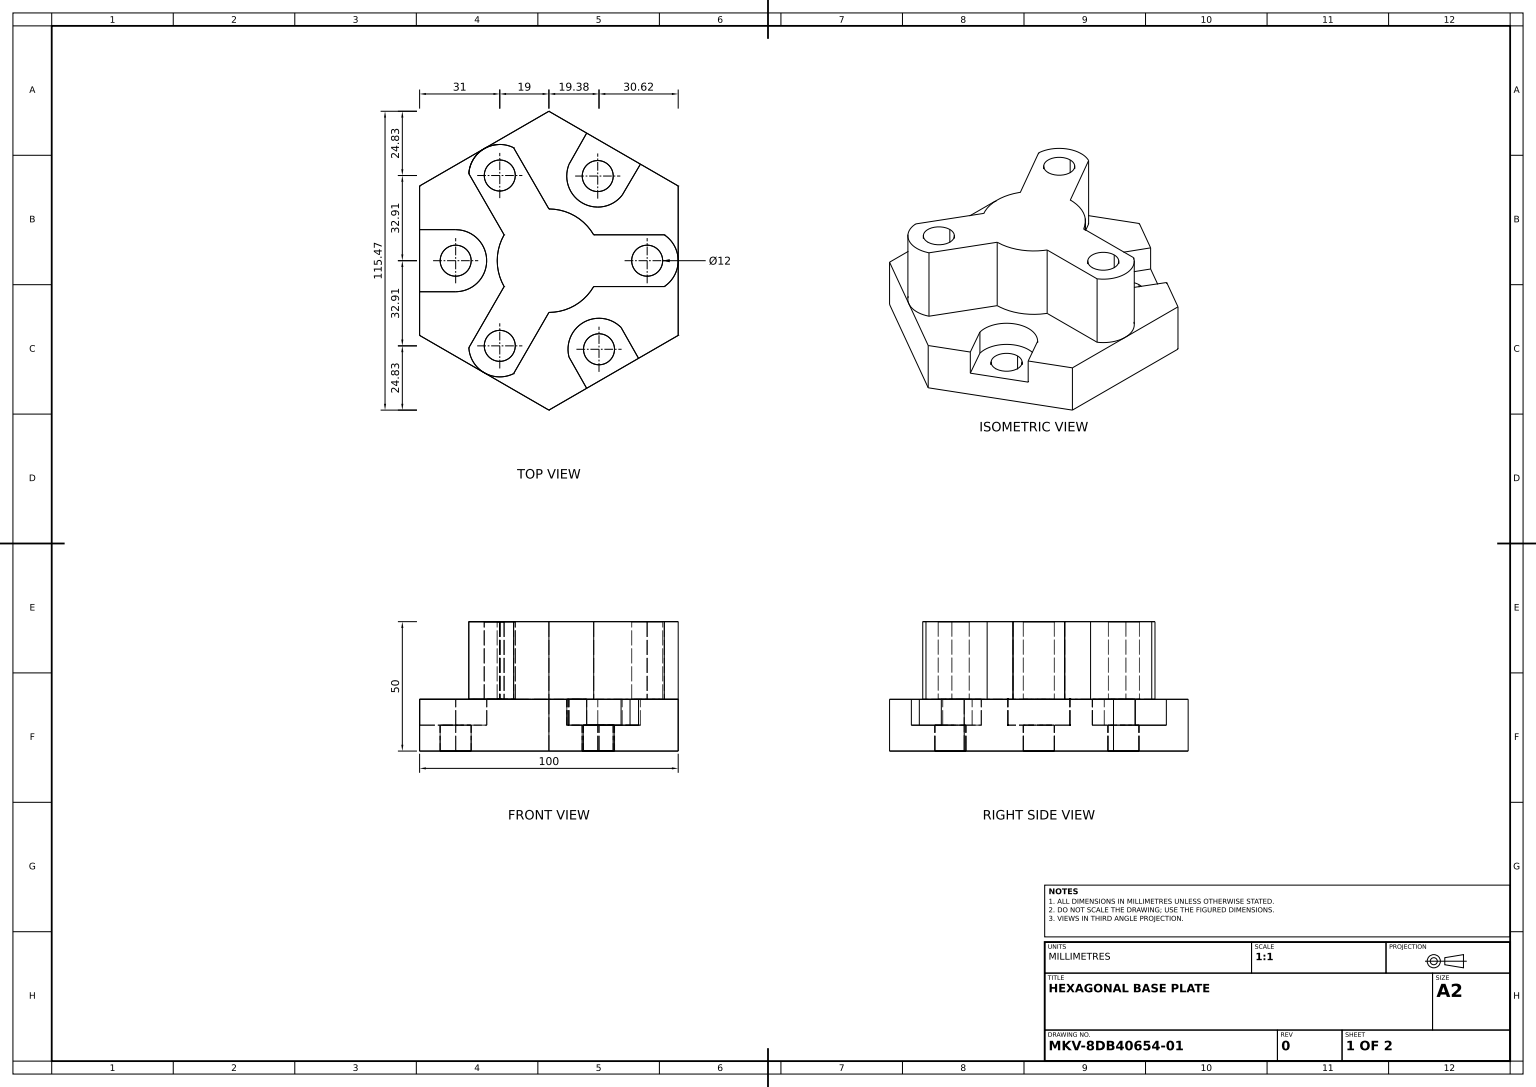
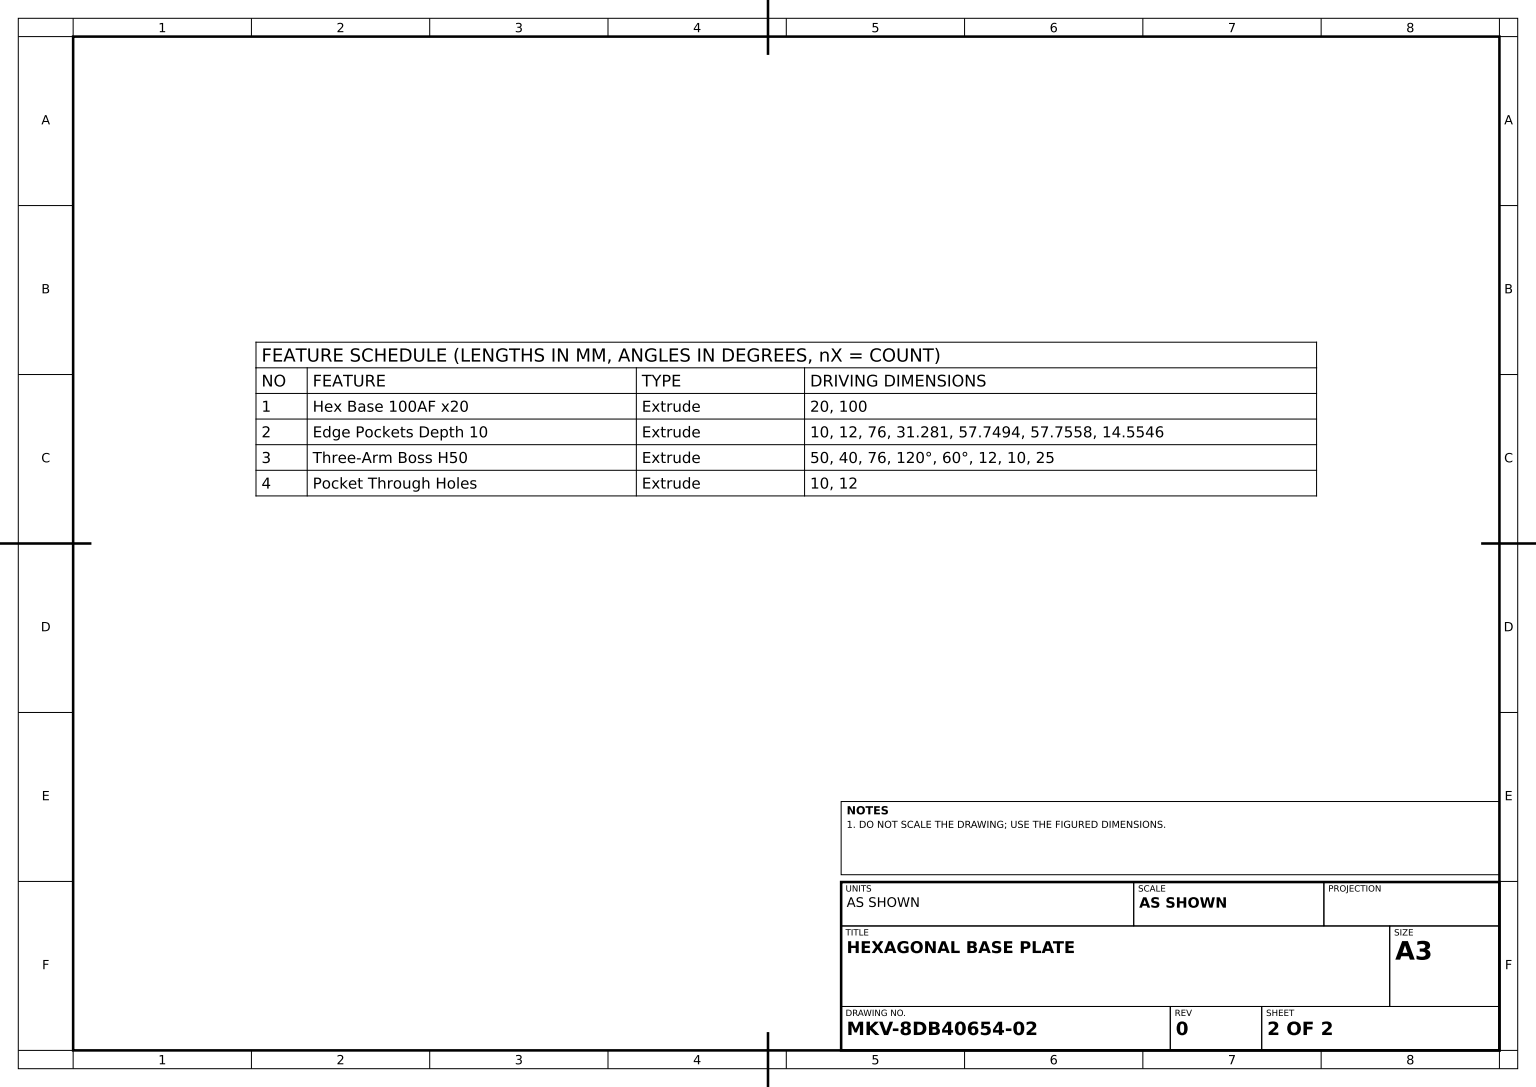
from build123d import *

# Parameters (mm, degrees)
HEX_BASE_100AF_X20_DEPTH    = 20
EDGE_POCKET_SKETCH_R        = 6
EDGE_POCKETS_DEPTH_10_DEPTH = 10
THREE_ARM_BOSS_SKETCH_R     = 6
THREE_ARM_BOSS_H50_DEPTH    = 50
POCKET_HOLE_SKETCH_R        = 6
POCKET_THROUGH_HOLES_DEPTH  = 10


with BuildPart() as part:
    # Hex Base Sketch → Hex Base 100AF x20 (new body)
    with BuildSketch(Plane(origin=(0, 0, 0), x_dir=(1, 0, 0), z_dir=(0, 1, 0))):
        Polygon((0, 57.735026919), (-50, 28.867513459), (-50, -28.867513459), (0, -57.735026919), (50, -28.867513459), (50, 28.867513459), align=None)
    extrude(amount=HEX_BASE_100AF_X20_DEPTH)

    # Edge Pocket Sketch → Edge Pockets Depth 10 (cut)
    # profile 1 of 6: a face of its own
    with BuildSketch(Plane(origin=(0, 20, 0), x_dir=(1, 0, 0), z_dir=(0, 1, 0))):
        with BuildLine():
            Line((-50, 12), (-50, -12))
            Line((-50, -12), (-36.055514092, -12))
            ThreePointArc((-36.055514092, -12), (-24.055514092, 0), (-36.055514092, 12))
            Line((-36.055514092, 12), (-50, 12))
        make_face()
        with Locations((-38.000001269, 0)):
            Circle(EDGE_POCKET_SKETCH_R, mode=Mode.SUBTRACT)
    # profile 2 of 6: a face of its own
    with BuildSketch(Plane(origin=(0, 20, 0), x_dir=(1, 0, 0), z_dir=(0, 1, 0))):
        with BuildLine():
            Line((35.392304845, 37.301270189), (14.607695155, 49.301270189))
            Line((14.607695155, 49.301270189), (7.755802012, 37.200102575))
            ThreePointArc((7.755802012, 37.200102575), (12.881704296, 22.311766329), (28.338332848, 25.316772856))
            Line((28.338332848, 25.316772856), (35.392304845, 37.301270189))
        make_face()
        with Locations((19.000000635, 32.908966443)):
            Circle(EDGE_POCKET_SKETCH_R, mode=Mode.SUBTRACT)
    # profile 3 of 6: a face of its own
    with BuildSketch(Plane(origin=(0, 20, 0), x_dir=(1, 0, 0), z_dir=(0, 1, 0))):
        with BuildLine():
            ThreePointArc((27.907341935, -25.791090759), (21.025211471, -22.343578273), (13.464344244, -23.786612875))
            ThreePointArc((13.464344244, -23.786612875), (8.335672837, -29.526455354), (7.749398434, -37.201437074))
            Line((7.749398434, -37.201437074), (8.639996816, -38.774801402))
            Line((8.639996816, -38.774801402), (14.600745568, -49.305282535))
            Line((14.600745568, -49.305282535), (34.661483865, -37.723209879))
            Line((34.661483865, -37.723209879), (28.797940317, -27.364455088))
            Line((28.797940317, -27.364455088), (27.907341935, -25.791090759))
        make_face()
        with BuildLine():
            ThreePointArc((24.718968567, -33.069628245), (15.696863266, -38.252955318), (15.763342049, -27.84810817))
            ThreePointArc((15.763342049, -27.84810817), (21.741073867, -27.886301171), (24.718968567, -33.069628245))
        make_face(mode=Mode.SUBTRACT)
    # profile 4 of 6: a face of its own
    with BuildSketch(Plane(origin=(0, 20, 0), x_dir=(1, 0, 0), z_dir=(0, 1, 0))):
        with Locations((18.718968567, -33.069628245)):
            Circle(EDGE_POCKET_SKETCH_R)
    # profile 5 of 6: a face of its own
    with BuildSketch(Plane(origin=(0, 20, 0), x_dir=(1, 0, 0), z_dir=(0, 1, 0))):
        with Locations((-38.000001269, 0)):
            Circle(EDGE_POCKET_SKETCH_R)
    # profile 6 of 6: a face of its own
    with BuildSketch(Plane(origin=(0, 20, 0), x_dir=(1, 0, 0), z_dir=(0, 1, 0))):
        with Locations((19.000000635, 32.908966443)):
            Circle(EDGE_POCKET_SKETCH_R)
    extrude(amount=-EDGE_POCKETS_DEPTH_10_DEPTH, mode=Mode.SUBTRACT)

    # Three-Arm Boss Sketch → Three-Arm Boss H50 (add)
    # profile 1 of 2: a face of its own
    with BuildSketch(Plane(origin=(0, 0, 0), x_dir=(1, 0, 0), z_dir=(0, 1, 0))):
        with BuildLine():
            ThreePointArc((0, -20), (10, -17.320508076), (17.320508076, -10))
            Line((17.320508076, -10), (25, -10))
            Line((25, -10), (25, 10))
            Line((25, 10), (17.320508076, 10))
            ThreePointArc((17.320508076, 10), (10, 17.320508076), (0, 20))
            Line((0, 20), (-13.656370753, 43.65352799))
            ThreePointArc((-13.656370753, 43.65352799), (-25, 43.301270189), (-30.976878828, 33.65352799))
            Line((-30.976878828, 33.65352799), (-17.320508076, 10))
            ThreePointArc((-17.320508076, 10), (-20, 0), (-17.320508076, -10))
            Line((-17.320508076, -10), (-30.976878828, -33.65352799))
            ThreePointArc((-30.976878828, -33.65352799), (-25, -43.301270189), (-13.656370753, -43.65352799))
            Line((-13.656370753, -43.65352799), (0, -20))
        make_face()
        with Locations(Location((-19, -32.908965344, 0), (0, 0, 270))):
            Circle(THREE_ARM_BOSS_SKETCH_R, mode=Mode.SUBTRACT)
        with Locations(Location((-19, 32.908965344, 0), (0, 0, 270))):
            Circle(THREE_ARM_BOSS_SKETCH_R, mode=Mode.SUBTRACT)
    # profile 2 of 2: a face of its own
    with BuildSketch(Plane(origin=(0, 0, 0), x_dir=(1, 0, 0), z_dir=(0, 1, 0))):
        with BuildLine():
            Line((25, 10), (25, -10))
            Line((25, -10), (44.633249581, -10))
            ThreePointArc((44.633249581, -10), (50, 0), (44.633249581, 10))
            Line((44.633249581, 10), (25, 10))
        make_face()
        with Locations(Location((38, 0, 0), (0, 0, 270))):
            Circle(THREE_ARM_BOSS_SKETCH_R, mode=Mode.SUBTRACT)
    extrude(amount=THREE_ARM_BOSS_H50_DEPTH)

    # Pocket Hole Sketch → Pocket Through Holes (cut)
    with BuildSketch(Plane(origin=(0, 10, 0), x_dir=(1, 0, 0), z_dir=(0, 1, 0))):
        with Locations(Location((19.375597278, -34.229653025, 0), (0, 0, 270))):
            Circle(POCKET_HOLE_SKETCH_R)
        with Locations(Location((-36.055514092, 0, 0), (0, 0, 270))):
            Circle(POCKET_HOLE_SKETCH_R)
        with Locations(Location((18.881704296, 32.704071174, 0), (0, 0, 270))):
            Circle(POCKET_HOLE_SKETCH_R)
    extrude(amount=-POCKET_THROUGH_HOLES_DEPTH, mode=Mode.SUBTRACT)


solid = part.part
